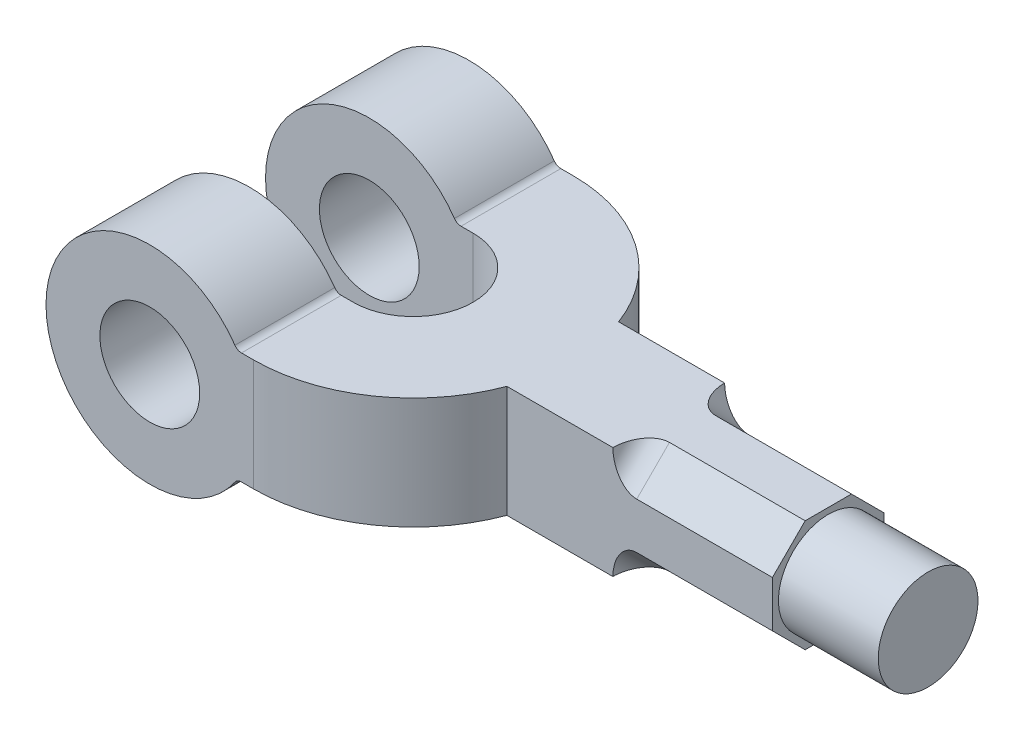
ISO-10303-21;
HEADER;
FILE_DESCRIPTION(('STEP AP214'),'2;1');
FILE_NAME('part.step','',(''),(''),'','','');
FILE_SCHEMA(('AUTOMOTIVE_DESIGN { 1 0 10303 214 1 1 1 1 }'));
ENDSEC;
DATA;
#1=APPLICATION_CONTEXT('core data for automotive mechanical design processes');
#2=APPLICATION_PROTOCOL_DEFINITION('international standard','automotive_design',2000,#1);
#3=PRODUCT_CONTEXT('',#1,'mechanical');
#4=PRODUCT('Part','Part','',(#3));
#5=PRODUCT_RELATED_PRODUCT_CATEGORY('part','',(#4));
#6=PRODUCT_DEFINITION_FORMATION('','',#4);
#7=PRODUCT_DEFINITION_CONTEXT('part definition',#1,'design');
#8=PRODUCT_DEFINITION('design','',#6,#7);
#9=PRODUCT_DEFINITION_SHAPE('','',#8);
#10=(LENGTH_UNIT() NAMED_UNIT(*) SI_UNIT(.MILLI.,.METRE.));
#11=(NAMED_UNIT(*) PLANE_ANGLE_UNIT() SI_UNIT($,.RADIAN.));
#12=(NAMED_UNIT(*) SI_UNIT($,.STERADIAN.) SOLID_ANGLE_UNIT());
#13=UNCERTAINTY_MEASURE_WITH_UNIT(LENGTH_MEASURE(1.E-05),#10,'distance_accuracy_value','');
#14=(GEOMETRIC_REPRESENTATION_CONTEXT(3) GLOBAL_UNCERTAINTY_ASSIGNED_CONTEXT((#13)) GLOBAL_UNIT_ASSIGNED_CONTEXT((#10,
#11,#12)) REPRESENTATION_CONTEXT('',''));
#15=CARTESIAN_POINT('',(0.,0.,0.));
#16=DIRECTION('',(0.,0.,1.));
#17=DIRECTION('',(1.,0.,0.));
#18=AXIS2_PLACEMENT_3D('',#15,#16,#17);
#19=CARTESIAN_POINT('',(-26.001,14.,-15.));
#20=DIRECTION('',(0.,-1.,0.));
#21=DIRECTION('',(0.,0.,-1.));
#22=AXIS2_PLACEMENT_3D('',#19,#20,#21);
#23=PLANE('',#22);
#24=DIRECTION('',(1.,0.,0.));
#25=VECTOR('',#24,1.);
#26=CARTESIAN_POINT('',(-26.001,14.,-40.));
#27=LINE('',#26,#25);
#28=CARTESIAN_POINT('',(22.9782505861521,14.,-40.));
#29=VERTEX_POINT('',#28);
#30=CARTESIAN_POINT('',(26.,14.,-40.));
#31=VERTEX_POINT('',#30);
#32=EDGE_CURVE('E276',#29,#31,#27,.T.);
#33=ORIENTED_EDGE('',*,*,#32,.F.);
#34=DIRECTION('',(0.,0.,1.));
#35=VECTOR('',#34,1.);
#36=CARTESIAN_POINT('',(22.9782505861521,14.,-15.));
#37=LINE('',#36,#35);
#38=CARTESIAN_POINT('',(22.9782505861521,14.,-15.));
#39=VERTEX_POINT('',#38);
#40=EDGE_CURVE('E344',#29,#39,#37,.T.);
#41=ORIENTED_EDGE('',*,*,#40,.T.);
#42=DIRECTION('',(1.,0.,0.));
#43=VECTOR('',#42,1.);
#44=CARTESIAN_POINT('',(-26.001,14.,-15.));
#45=LINE('',#44,#43);
#46=CARTESIAN_POINT('',(26.,14.,-15.));
#47=VERTEX_POINT('',#46);
#48=EDGE_CURVE('E274',#39,#47,#45,.T.);
#49=ORIENTED_EDGE('',*,*,#48,.T.);
#50=CARTESIAN_POINT('',(26.,14.,0.));
#51=DIRECTION('',(0.,-1.,0.));
#52=DIRECTION('',(0.,0.,1.));
#53=AXIS2_PLACEMENT_3D('',#50,#51,#52);
#54=CIRCLE('',#53,15.);
#55=CARTESIAN_POINT('',(26.,14.,15.));
#56=VERTEX_POINT('',#55);
#57=EDGE_CURVE('E238',#47,#56,#54,.T.);
#58=ORIENTED_EDGE('',*,*,#57,.T.);
#59=DIRECTION('',(1.,0.,0.));
#60=VECTOR('',#59,1.);
#61=CARTESIAN_POINT('',(-26.001,14.,15.));
#62=LINE('',#61,#60);
#63=CARTESIAN_POINT('',(22.9782505861521,14.,15.));
#64=VERTEX_POINT('',#63);
#65=EDGE_CURVE('E414',#64,#56,#62,.T.);
#66=ORIENTED_EDGE('',*,*,#65,.F.);
#67=DIRECTION('',(0.,0.,1.));
#68=VECTOR('',#67,1.);
#69=CARTESIAN_POINT('',(22.9782505861521,14.,40.));
#70=LINE('',#69,#68);
#71=CARTESIAN_POINT('',(22.9782505861521,14.,40.));
#72=VERTEX_POINT('',#71);
#73=EDGE_CURVE('E54',#64,#72,#70,.T.);
#74=ORIENTED_EDGE('',*,*,#73,.T.);
#75=DIRECTION('',(1.,0.,0.));
#76=VECTOR('',#75,1.);
#77=CARTESIAN_POINT('',(-26.001,14.,40.));
#78=LINE('',#77,#76);
#79=CARTESIAN_POINT('',(26.,14.,40.));
#80=VERTEX_POINT('',#79);
#81=EDGE_CURVE('E246',#72,#80,#78,.T.);
#82=ORIENTED_EDGE('',*,*,#81,.T.);
#83=CARTESIAN_POINT('',(26.,14.,0.));
#84=DIRECTION('',(0.,1.,0.));
#85=DIRECTION('',(0.,0.,1.));
#86=AXIS2_PLACEMENT_3D('',#83,#84,#85);
#87=CIRCLE('',#86,40.);
#88=CARTESIAN_POINT('',(63.4699879903904,14.,14.));
#89=VERTEX_POINT('',#88);
#90=EDGE_CURVE('E235',#80,#89,#87,.T.);
#91=ORIENTED_EDGE('',*,*,#90,.T.);
#92=DIRECTION('',(1.,0.,0.));
#93=VECTOR('',#92,1.);
#94=CARTESIAN_POINT('',(130.,14.,14.));
#95=LINE('',#94,#93);
#96=CARTESIAN_POINT('',(90.0033680345603,14.,14.));
#97=VERTEX_POINT('',#96);
#98=EDGE_CURVE('E226',#89,#97,#95,.T.);
#99=ORIENTED_EDGE('',*,*,#98,.T.);
#100=CARTESIAN_POINT('',(96.,14.,14.2842712474619));
#101=DIRECTION('',(0.,-1.,0.));
#102=DIRECTION('',(0.,0.,-1.));
#103=AXIS2_PLACEMENT_3D('',#100,#101,#102);
#104=ELLIPSE('',#103,8.48528137423856,6.);
#105=CARTESIAN_POINT('',(96.,14.,5.79898987322334));
#106=VERTEX_POINT('',#105);
#107=EDGE_CURVE('E319',#97,#106,#104,.T.);
#108=ORIENTED_EDGE('',*,*,#107,.T.);
#109=DIRECTION('',(1.,0.,0.));
#110=VECTOR('',#109,1.);
#111=CARTESIAN_POINT('',(90.,14.,5.79898987322334));
#112=LINE('',#111,#110);
#113=CARTESIAN_POINT('',(130.,14.,5.79898987322334));
#114=VERTEX_POINT('',#113);
#115=EDGE_CURVE('E208',#106,#114,#112,.T.);
#116=ORIENTED_EDGE('',*,*,#115,.T.);
#117=DIRECTION('',(0.,0.,-1.));
#118=VECTOR('',#117,1.);
#119=CARTESIAN_POINT('',(130.,14.,-14.));
#120=LINE('',#119,#118);
#121=CARTESIAN_POINT('',(130.,14.,-5.79898987322332));
#122=VERTEX_POINT('',#121);
#123=EDGE_CURVE('E219',#114,#122,#120,.T.);
#124=ORIENTED_EDGE('',*,*,#123,.T.);
#125=DIRECTION('',(1.,0.,0.));
#126=VECTOR('',#125,1.);
#127=CARTESIAN_POINT('',(90.,14.,-5.79898987322332));
#128=LINE('',#127,#126);
#129=CARTESIAN_POINT('',(96.,14.,-5.79898987322332));
#130=VERTEX_POINT('',#129);
#131=EDGE_CURVE('E200',#130,#122,#128,.T.);
#132=ORIENTED_EDGE('',*,*,#131,.F.);
#133=CARTESIAN_POINT('',(96.,14.,-14.2842712474619));
#134=DIRECTION('',(0.,-1.,0.));
#135=DIRECTION('',(0.,0.,-1.));
#136=AXIS2_PLACEMENT_3D('',#133,#134,#135);
#137=ELLIPSE('',#136,8.48528137423857,6.);
#138=CARTESIAN_POINT('',(90.0033680345603,14.,-14.));
#139=VERTEX_POINT('',#138);
#140=EDGE_CURVE('E311',#130,#139,#137,.T.);
#141=ORIENTED_EDGE('',*,*,#140,.T.);
#142=DIRECTION('',(-1.,0.,0.));
#143=VECTOR('',#142,1.);
#144=CARTESIAN_POINT('',(130.,14.,-14.));
#145=LINE('',#144,#143);
#146=CARTESIAN_POINT('',(63.4699879903904,14.,-14.));
#147=VERTEX_POINT('',#146);
#148=EDGE_CURVE('E227',#139,#147,#145,.T.);
#149=ORIENTED_EDGE('',*,*,#148,.T.);
#150=CARTESIAN_POINT('',(26.,14.,0.));
#151=DIRECTION('',(0.,1.,0.));
#152=DIRECTION('',(0.,0.,1.));
#153=AXIS2_PLACEMENT_3D('',#150,#151,#152);
#154=CIRCLE('',#153,40.);
#155=EDGE_CURVE('E229',#147,#31,#154,.T.);
#156=ORIENTED_EDGE('',*,*,#155,.T.);
#157=EDGE_LOOP('',(#33,#41,#49,#58,#66,#74,#82,#91,#99,#108,#116,#124,#132,#141,#149,#156));
#158=FACE_BOUND('',#157,.T.);
#159=ADVANCED_FACE('F37',(#158),#23,.F.);
#160=CARTESIAN_POINT('',(130.,14.,14.));
#161=DIRECTION('',(0.,0.,-1.));
#162=DIRECTION('',(-1.,0.,0.));
#163=AXIS2_PLACEMENT_3D('',#160,#161,#162);
#164=PLANE('',#163);
#165=DIRECTION('',(1.,0.,0.));
#166=VECTOR('',#165,1.);
#167=CARTESIAN_POINT('',(130.,-14.,14.));
#168=LINE('',#167,#166);
#169=CARTESIAN_POINT('',(63.4699879903904,-14.,14.));
#170=VERTEX_POINT('',#169);
#171=CARTESIAN_POINT('',(90.0033680345603,-14.,14.));
#172=VERTEX_POINT('',#171);
#173=EDGE_CURVE('E244',#170,#172,#168,.T.);
#174=ORIENTED_EDGE('',*,*,#173,.T.);
#175=CARTESIAN_POINT('',(96.,-14.2842712474619,14.));
#176=DIRECTION('',(0.,0.,-1.));
#177=DIRECTION('',(0.,1.,0.));
#178=AXIS2_PLACEMENT_3D('',#175,#176,#177);
#179=ELLIPSE('',#178,8.48528137423857,6.);
#180=CARTESIAN_POINT('',(96.,-5.79898987322333,14.));
#181=VERTEX_POINT('',#180);
#182=EDGE_CURVE('E324',#172,#181,#179,.T.);
#183=ORIENTED_EDGE('',*,*,#182,.T.);
#184=DIRECTION('',(1.,0.,0.));
#185=VECTOR('',#184,1.);
#186=CARTESIAN_POINT('',(90.,-5.79898987322333,14.));
#187=LINE('',#186,#185);
#188=CARTESIAN_POINT('',(130.,-5.79898987322333,14.));
#189=VERTEX_POINT('',#188);
#190=EDGE_CURVE('E432',#181,#189,#187,.T.);
#191=ORIENTED_EDGE('',*,*,#190,.T.);
#192=DIRECTION('',(0.,-1.,0.));
#193=VECTOR('',#192,1.);
#194=CARTESIAN_POINT('',(130.,14.,14.));
#195=LINE('',#194,#193);
#196=CARTESIAN_POINT('',(130.,5.79898987322333,14.));
#197=VERTEX_POINT('',#196);
#198=EDGE_CURVE('E269',#197,#189,#195,.T.);
#199=ORIENTED_EDGE('',*,*,#198,.F.);
#200=DIRECTION('',(1.,0.,0.));
#201=VECTOR('',#200,1.);
#202=CARTESIAN_POINT('',(90.,5.79898987322332,14.));
#203=LINE('',#202,#201);
#204=CARTESIAN_POINT('',(96.,5.79898987322332,14.));
#205=VERTEX_POINT('',#204);
#206=EDGE_CURVE('E430',#205,#197,#203,.T.);
#207=ORIENTED_EDGE('',*,*,#206,.F.);
#208=CARTESIAN_POINT('',(96.,14.2842712474619,14.));
#209=DIRECTION('',(0.,0.,-1.));
#210=DIRECTION('',(0.,1.,0.));
#211=AXIS2_PLACEMENT_3D('',#208,#209,#210);
#212=ELLIPSE('',#211,8.48528137423857,6.);
#213=EDGE_CURVE('E314',#205,#97,#212,.T.);
#214=ORIENTED_EDGE('',*,*,#213,.T.);
#215=ORIENTED_EDGE('',*,*,#98,.F.);
#216=DIRECTION('',(0.,-1.,0.));
#217=VECTOR('',#216,1.);
#218=CARTESIAN_POINT('',(63.4699879903904,14.,14.));
#219=LINE('',#218,#217);
#220=EDGE_CURVE('E272',#89,#170,#219,.T.);
#221=ORIENTED_EDGE('',*,*,#220,.T.);
#222=EDGE_LOOP('',(#174,#183,#191,#199,#207,#214,#215,#221));
#223=FACE_BOUND('',#222,.T.);
#224=ADVANCED_FACE('F421',(#223),#164,.F.);
#225=CARTESIAN_POINT('',(130.,14.,-14.));
#226=DIRECTION('',(-1.,0.,0.));
#227=DIRECTION('',(0.,0.,1.));
#228=AXIS2_PLACEMENT_3D('',#225,#226,#227);
#229=PLANE('',#228);
#230=CARTESIAN_POINT('',(130.,0.,0.));
#231=DIRECTION('',(1.,0.,0.));
#232=DIRECTION('',(0.,0.,-1.));
#233=AXIS2_PLACEMENT_3D('',#230,#231,#232);
#234=CIRCLE('',#233,12.5);
#235=CARTESIAN_POINT('',(130.,0.,-12.5));
#236=VERTEX_POINT('',#235);
#237=EDGE_CURVE('E323',#236,#236,#234,.T.);
#238=ORIENTED_EDGE('',*,*,#237,.F.);
#239=EDGE_LOOP('',(#238));
#240=FACE_BOUND('',#239,.T.);
#241=DIRECTION('',(0.,0.707106781186548,-0.707106781186547));
#242=VECTOR('',#241,1.);
#243=CARTESIAN_POINT('',(130.,-14.,-5.79898987322333));
#244=LINE('',#243,#242);
#245=CARTESIAN_POINT('',(130.,-14.,-5.79898987322333));
#246=VERTEX_POINT('',#245);
#247=CARTESIAN_POINT('',(130.,-5.79898987322332,-14.));
#248=VERTEX_POINT('',#247);
#249=EDGE_CURVE('E225',#246,#248,#244,.T.);
#250=ORIENTED_EDGE('',*,*,#249,.T.);
#251=DIRECTION('',(0.,-1.,0.));
#252=VECTOR('',#251,1.);
#253=CARTESIAN_POINT('',(130.,14.,-14.));
#254=LINE('',#253,#252);
#255=CARTESIAN_POINT('',(130.,5.79898987322333,-14.));
#256=VERTEX_POINT('',#255);
#257=EDGE_CURVE('E220',#256,#248,#254,.T.);
#258=ORIENTED_EDGE('',*,*,#257,.F.);
#259=DIRECTION('',(0.,0.707106781186547,0.707106781186548));
#260=VECTOR('',#259,1.);
#261=CARTESIAN_POINT('',(130.,5.79898987322333,-14.));
#262=LINE('',#261,#260);
#263=EDGE_CURVE('E201',#256,#122,#262,.T.);
#264=ORIENTED_EDGE('',*,*,#263,.T.);
#265=ORIENTED_EDGE('',*,*,#123,.F.);
#266=DIRECTION('',(0.,-0.707106781186548,0.707106781186547));
#267=VECTOR('',#266,1.);
#268=CARTESIAN_POINT('',(130.,14.,5.79898987322334));
#269=LINE('',#268,#267);
#270=EDGE_CURVE('E222',#114,#197,#269,.T.);
#271=ORIENTED_EDGE('',*,*,#270,.T.);
#272=ORIENTED_EDGE('',*,*,#198,.T.);
#273=DIRECTION('',(0.,-0.707106781186547,-0.707106781186548));
#274=VECTOR('',#273,1.);
#275=CARTESIAN_POINT('',(130.,-5.79898987322333,14.));
#276=LINE('',#275,#274);
#277=CARTESIAN_POINT('',(130.,-14.,5.79898987322333));
#278=VERTEX_POINT('',#277);
#279=EDGE_CURVE('E437',#189,#278,#276,.T.);
#280=ORIENTED_EDGE('',*,*,#279,.T.);
#281=DIRECTION('',(0.,0.,-1.));
#282=VECTOR('',#281,1.);
#283=CARTESIAN_POINT('',(130.,-14.,-14.));
#284=LINE('',#283,#282);
#285=EDGE_CURVE('E247',#278,#246,#284,.T.);
#286=ORIENTED_EDGE('',*,*,#285,.T.);
#287=EDGE_LOOP('',(#250,#258,#264,#265,#271,#272,#280,#286));
#288=FACE_BOUND('',#287,.T.);
#289=ADVANCED_FACE('F216',(#240,#288),#229,.F.);
#290=CARTESIAN_POINT('',(130.,14.,-14.));
#291=DIRECTION('',(0.,0.,1.));
#292=DIRECTION('',(1.,0.,0.));
#293=AXIS2_PLACEMENT_3D('',#290,#291,#292);
#294=PLANE('',#293);
#295=DIRECTION('',(1.,0.,0.));
#296=VECTOR('',#295,1.);
#297=CARTESIAN_POINT('',(90.,-5.79898987322332,-14.));
#298=LINE('',#297,#296);
#299=CARTESIAN_POINT('',(96.,-5.79898987322332,-14.));
#300=VERTEX_POINT('',#299);
#301=EDGE_CURVE('E438',#300,#248,#298,.T.);
#302=ORIENTED_EDGE('',*,*,#301,.F.);
#303=CARTESIAN_POINT('',(96.,-14.2842712474619,-14.));
#304=DIRECTION('',(0.,0.,1.));
#305=DIRECTION('',(0.,-1.,0.));
#306=AXIS2_PLACEMENT_3D('',#303,#304,#305);
#307=ELLIPSE('',#306,8.48528137423857,6.);
#308=CARTESIAN_POINT('',(90.0033680345603,-14.,-14.));
#309=VERTEX_POINT('',#308);
#310=EDGE_CURVE('E306',#300,#309,#307,.T.);
#311=ORIENTED_EDGE('',*,*,#310,.T.);
#312=DIRECTION('',(-1.,0.,0.));
#313=VECTOR('',#312,1.);
#314=CARTESIAN_POINT('',(130.,-14.,-14.));
#315=LINE('',#314,#313);
#316=CARTESIAN_POINT('',(63.4699879903904,-14.,-14.));
#317=VERTEX_POINT('',#316);
#318=EDGE_CURVE('E252',#309,#317,#315,.T.);
#319=ORIENTED_EDGE('',*,*,#318,.T.);
#320=DIRECTION('',(0.,-1.,0.));
#321=VECTOR('',#320,1.);
#322=CARTESIAN_POINT('',(63.4699879903904,14.,-14.));
#323=LINE('',#322,#321);
#324=EDGE_CURVE('E263',#147,#317,#323,.T.);
#325=ORIENTED_EDGE('',*,*,#324,.F.);
#326=ORIENTED_EDGE('',*,*,#148,.F.);
#327=CARTESIAN_POINT('',(96.,14.2842712474619,-14.));
#328=DIRECTION('',(0.,0.,1.));
#329=DIRECTION('',(0.,-1.,0.));
#330=AXIS2_PLACEMENT_3D('',#327,#328,#329);
#331=ELLIPSE('',#330,8.48528137423857,6.);
#332=CARTESIAN_POINT('',(96.,5.79898987322333,-14.));
#333=VERTEX_POINT('',#332);
#334=EDGE_CURVE('E312',#139,#333,#331,.T.);
#335=ORIENTED_EDGE('',*,*,#334,.T.);
#336=DIRECTION('',(1.,0.,0.));
#337=VECTOR('',#336,1.);
#338=CARTESIAN_POINT('',(90.,5.79898987322333,-14.));
#339=LINE('',#338,#337);
#340=EDGE_CURVE('E212',#333,#256,#339,.T.);
#341=ORIENTED_EDGE('',*,*,#340,.T.);
#342=ORIENTED_EDGE('',*,*,#257,.T.);
#343=EDGE_LOOP('',(#302,#311,#319,#325,#326,#335,#341,#342));
#344=FACE_BOUND('',#343,.T.);
#345=ADVANCED_FACE('F458',(#344),#294,.F.);
#346=CARTESIAN_POINT('',(26.,-14.,0.));
#347=DIRECTION('',(0.,1.,0.));
#348=DIRECTION('',(0.,0.,1.));
#349=AXIS2_PLACEMENT_3D('',#346,#347,#348);
#350=PLANE('',#349);
#351=DIRECTION('',(1.,0.,0.));
#352=VECTOR('',#351,1.);
#353=CARTESIAN_POINT('',(-26.001,-14.,-15.));
#354=LINE('',#353,#352);
#355=CARTESIAN_POINT('',(22.9782505861521,-14.,-15.));
#356=VERTEX_POINT('',#355);
#357=CARTESIAN_POINT('',(26.,-14.,-15.));
#358=VERTEX_POINT('',#357);
#359=EDGE_CURVE('E384',#356,#358,#354,.T.);
#360=ORIENTED_EDGE('',*,*,#359,.F.);
#361=DIRECTION('',(0.,0.,1.));
#362=VECTOR('',#361,1.);
#363=CARTESIAN_POINT('',(22.9782505861521,-14.,-40.));
#364=LINE('',#363,#362);
#365=CARTESIAN_POINT('',(22.9782505861521,-14.,-40.));
#366=VERTEX_POINT('',#365);
#367=EDGE_CURVE('E331',#356,#366,#364,.F.);
#368=ORIENTED_EDGE('',*,*,#367,.T.);
#369=DIRECTION('',(1.,0.,0.));
#370=VECTOR('',#369,1.);
#371=CARTESIAN_POINT('',(-26.001,-14.,-40.));
#372=LINE('',#371,#370);
#373=CARTESIAN_POINT('',(26.,-14.,-40.));
#374=VERTEX_POINT('',#373);
#375=EDGE_CURVE('E378',#366,#374,#372,.T.);
#376=ORIENTED_EDGE('',*,*,#375,.T.);
#377=CARTESIAN_POINT('',(26.,-14.,0.));
#378=DIRECTION('',(0.,1.,0.));
#379=DIRECTION('',(0.,0.,1.));
#380=AXIS2_PLACEMENT_3D('',#377,#378,#379);
#381=CIRCLE('',#380,40.);
#382=EDGE_CURVE('E254',#317,#374,#381,.T.);
#383=ORIENTED_EDGE('',*,*,#382,.F.);
#384=ORIENTED_EDGE('',*,*,#318,.F.);
#385=CARTESIAN_POINT('',(96.,-14.,-14.2842712474619));
#386=DIRECTION('',(0.,1.,0.));
#387=DIRECTION('',(0.,0.,1.));
#388=AXIS2_PLACEMENT_3D('',#385,#386,#387);
#389=ELLIPSE('',#388,8.48528137423857,6.);
#390=CARTESIAN_POINT('',(96.,-14.,-5.79898987322333));
#391=VERTEX_POINT('',#390);
#392=EDGE_CURVE('E307',#309,#391,#389,.T.);
#393=ORIENTED_EDGE('',*,*,#392,.T.);
#394=DIRECTION('',(1.,0.,0.));
#395=VECTOR('',#394,1.);
#396=CARTESIAN_POINT('',(90.,-14.,-5.79898987322333));
#397=LINE('',#396,#395);
#398=EDGE_CURVE('E392',#391,#246,#397,.T.);
#399=ORIENTED_EDGE('',*,*,#398,.T.);
#400=ORIENTED_EDGE('',*,*,#285,.F.);
#401=DIRECTION('',(1.,0.,0.));
#402=VECTOR('',#401,1.);
#403=CARTESIAN_POINT('',(90.,-14.,5.79898987322333));
#404=LINE('',#403,#402);
#405=CARTESIAN_POINT('',(96.,-14.,5.79898987322333));
#406=VERTEX_POINT('',#405);
#407=EDGE_CURVE('E393',#406,#278,#404,.T.);
#408=ORIENTED_EDGE('',*,*,#407,.F.);
#409=CARTESIAN_POINT('',(96.,-14.,14.2842712474619));
#410=DIRECTION('',(0.,1.,0.));
#411=DIRECTION('',(0.,0.,1.));
#412=AXIS2_PLACEMENT_3D('',#409,#410,#411);
#413=ELLIPSE('',#412,8.48528137423857,6.);
#414=EDGE_CURVE('E318',#406,#172,#413,.T.);
#415=ORIENTED_EDGE('',*,*,#414,.T.);
#416=ORIENTED_EDGE('',*,*,#173,.F.);
#417=CARTESIAN_POINT('',(26.,-14.,0.));
#418=DIRECTION('',(0.,1.,0.));
#419=DIRECTION('',(0.,0.,1.));
#420=AXIS2_PLACEMENT_3D('',#417,#418,#419);
#421=CIRCLE('',#420,40.);
#422=CARTESIAN_POINT('',(26.,-14.,40.));
#423=VERTEX_POINT('',#422);
#424=EDGE_CURVE('E245',#423,#170,#421,.T.);
#425=ORIENTED_EDGE('',*,*,#424,.F.);
#426=DIRECTION('',(1.,0.,0.));
#427=VECTOR('',#426,1.);
#428=CARTESIAN_POINT('',(-26.001,-14.,40.));
#429=LINE('',#428,#427);
#430=CARTESIAN_POINT('',(22.9782505861521,-14.,40.));
#431=VERTEX_POINT('',#430);
#432=EDGE_CURVE('E385',#431,#423,#429,.T.);
#433=ORIENTED_EDGE('',*,*,#432,.F.);
#434=DIRECTION('',(0.,0.,1.));
#435=VECTOR('',#434,1.);
#436=CARTESIAN_POINT('',(22.9782505861521,-14.,15.));
#437=LINE('',#436,#435);
#438=CARTESIAN_POINT('',(22.9782505861521,-14.,15.));
#439=VERTEX_POINT('',#438);
#440=EDGE_CURVE('E335',#431,#439,#437,.F.);
#441=ORIENTED_EDGE('',*,*,#440,.T.);
#442=DIRECTION('',(1.,0.,0.));
#443=VECTOR('',#442,1.);
#444=CARTESIAN_POINT('',(-26.001,-14.,15.));
#445=LINE('',#444,#443);
#446=CARTESIAN_POINT('',(26.,-14.,15.));
#447=VERTEX_POINT('',#446);
#448=EDGE_CURVE('E399',#439,#447,#445,.T.);
#449=ORIENTED_EDGE('',*,*,#448,.T.);
#450=CARTESIAN_POINT('',(26.,-14.,0.));
#451=DIRECTION('',(0.,-1.,0.));
#452=DIRECTION('',(0.,0.,1.));
#453=AXIS2_PLACEMENT_3D('',#450,#451,#452);
#454=CIRCLE('',#453,15.);
#455=EDGE_CURVE('E257',#358,#447,#454,.T.);
#456=ORIENTED_EDGE('',*,*,#455,.F.);
#457=EDGE_LOOP('',(#360,#368,#376,#383,#384,#393,#399,#400,#408,#415,#416,#425,#433,#441,#449,#456));
#458=FACE_BOUND('',#457,.T.);
#459=ADVANCED_FACE('F391',(#458),#350,.F.);
#460=CARTESIAN_POINT('',(0.,0.,40.));
#461=DIRECTION('',(0.,0.,-1.));
#462=DIRECTION('',(-1.,0.,0.));
#463=AXIS2_PLACEMENT_3D('',#460,#461,#462);
#464=CYLINDRICAL_SURFACE('',#463,26.);
#465=CARTESIAN_POINT('',(0.,0.,-40.));
#466=DIRECTION('',(0.,0.,1.));
#467=DIRECTION('',(1.,0.,0.));
#468=AXIS2_PLACEMENT_3D('',#465,#466,#467);
#469=CIRCLE('',#468,26.);
#470=CARTESIAN_POINT('',(21.3369469728555,14.8571428571429,-40.));
#471=VERTEX_POINT('',#470);
#472=CARTESIAN_POINT('',(21.3369469728555,-14.8571428571429,-40.));
#473=VERTEX_POINT('',#472);
#474=EDGE_CURVE('E279',#471,#473,#469,.T.);
#475=ORIENTED_EDGE('',*,*,#474,.T.);
#476=DIRECTION('',(0.,0.,-1.));
#477=VECTOR('',#476,1.);
#478=CARTESIAN_POINT('',(21.3369469728555,-14.8571428571429,40.));
#479=LINE('',#478,#477);
#480=CARTESIAN_POINT('',(21.3369469728555,-14.8571428571429,-15.));
#481=VERTEX_POINT('',#480);
#482=EDGE_CURVE('E328',#473,#481,#479,.F.);
#483=ORIENTED_EDGE('',*,*,#482,.T.);
#484=CARTESIAN_POINT('',(0.,0.,-15.));
#485=DIRECTION('',(0.,0.,1.));
#486=DIRECTION('',(1.,0.,0.));
#487=AXIS2_PLACEMENT_3D('',#484,#485,#486);
#488=CIRCLE('',#487,26.);
#489=CARTESIAN_POINT('',(21.3369469728555,14.8571428571429,-15.));
#490=VERTEX_POINT('',#489);
#491=EDGE_CURVE('E293',#490,#481,#488,.T.);
#492=ORIENTED_EDGE('',*,*,#491,.F.);
#493=DIRECTION('',(0.,0.,-1.));
#494=VECTOR('',#493,1.);
#495=CARTESIAN_POINT('',(21.3369469728555,14.8571428571429,40.));
#496=LINE('',#495,#494);
#497=EDGE_CURVE('E326',#490,#471,#496,.T.);
#498=ORIENTED_EDGE('',*,*,#497,.T.);
#499=EDGE_LOOP('',(#475,#483,#492,#498));
#500=FACE_BOUND('',#499,.T.);
#501=ADVANCED_FACE('F362',(#500),#464,.T.);
#502=CARTESIAN_POINT('',(0.,0.,40.));
#503=DIRECTION('',(0.,0.,-1.));
#504=DIRECTION('',(-1.,0.,0.));
#505=AXIS2_PLACEMENT_3D('',#502,#503,#504);
#506=CYLINDRICAL_SURFACE('',#505,26.);
#507=CARTESIAN_POINT('',(0.,0.,15.));
#508=DIRECTION('',(0.,0.,1.));
#509=DIRECTION('',(1.,0.,0.));
#510=AXIS2_PLACEMENT_3D('',#507,#508,#509);
#511=CIRCLE('',#510,26.);
#512=CARTESIAN_POINT('',(21.3369469728555,14.8571428571429,15.));
#513=VERTEX_POINT('',#512);
#514=CARTESIAN_POINT('',(21.3369469728555,-14.8571428571429,15.));
#515=VERTEX_POINT('',#514);
#516=EDGE_CURVE('E404',#513,#515,#511,.T.);
#517=ORIENTED_EDGE('',*,*,#516,.T.);
#518=DIRECTION('',(0.,0.,-1.));
#519=VECTOR('',#518,1.);
#520=CARTESIAN_POINT('',(21.3369469728555,-14.8571428571429,40.));
#521=LINE('',#520,#519);
#522=CARTESIAN_POINT('',(21.3369469728555,-14.8571428571429,40.));
#523=VERTEX_POINT('',#522);
#524=EDGE_CURVE('E339',#515,#523,#521,.F.);
#525=ORIENTED_EDGE('',*,*,#524,.T.);
#526=CARTESIAN_POINT('',(0.,0.,40.));
#527=DIRECTION('',(0.,0.,1.));
#528=DIRECTION('',(1.,0.,0.));
#529=AXIS2_PLACEMENT_3D('',#526,#527,#528);
#530=CIRCLE('',#529,26.);
#531=CARTESIAN_POINT('',(21.3369469728555,14.8571428571429,40.));
#532=VERTEX_POINT('',#531);
#533=EDGE_CURVE('E408',#532,#523,#530,.T.);
#534=ORIENTED_EDGE('',*,*,#533,.F.);
#535=DIRECTION('',(0.,0.,-1.));
#536=VECTOR('',#535,1.);
#537=CARTESIAN_POINT('',(21.3369469728555,14.8571428571429,40.));
#538=LINE('',#537,#536);
#539=EDGE_CURVE('E337',#532,#513,#538,.T.);
#540=ORIENTED_EDGE('',*,*,#539,.T.);
#541=EDGE_LOOP('',(#517,#525,#534,#540));
#542=FACE_BOUND('',#541,.T.);
#543=ADVANCED_FACE('F495',(#542),#506,.T.);
#544=CARTESIAN_POINT('',(0.,0.,40.));
#545=DIRECTION('',(0.,0.,-1.));
#546=DIRECTION('',(-1.,0.,0.));
#547=AXIS2_PLACEMENT_3D('',#544,#545,#546);
#548=CYLINDRICAL_SURFACE('',#547,12.5);
#549=CARTESIAN_POINT('',(0.,0.,-40.));
#550=DIRECTION('',(0.,0.,1.));
#551=DIRECTION('',(1.,0.,0.));
#552=AXIS2_PLACEMENT_3D('',#549,#550,#551);
#553=CIRCLE('',#552,12.5);
#554=CARTESIAN_POINT('',(12.5,0.,-40.));
#555=VERTEX_POINT('',#554);
#556=EDGE_CURVE('E289',#555,#555,#553,.T.);
#557=ORIENTED_EDGE('',*,*,#556,.F.);
#558=EDGE_LOOP('',(#557));
#559=FACE_BOUND('',#558,.T.);
#560=CARTESIAN_POINT('',(0.,0.,-15.));
#561=DIRECTION('',(0.,0.,1.));
#562=DIRECTION('',(1.,0.,0.));
#563=AXIS2_PLACEMENT_3D('',#560,#561,#562);
#564=CIRCLE('',#563,12.5);
#565=CARTESIAN_POINT('',(12.5,0.,-15.));
#566=VERTEX_POINT('',#565);
#567=EDGE_CURVE('E290',#566,#566,#564,.T.);
#568=ORIENTED_EDGE('',*,*,#567,.T.);
#569=EDGE_LOOP('',(#568));
#570=FACE_BOUND('',#569,.T.);
#571=ADVANCED_FACE('F488',(#559,#570),#548,.F.);
#572=CARTESIAN_POINT('',(0.,0.,-40.));
#573=DIRECTION('',(0.,0.,1.));
#574=DIRECTION('',(1.,0.,0.));
#575=AXIS2_PLACEMENT_3D('',#572,#573,#574);
#576=PLANE('',#575);
#577=ORIENTED_EDGE('',*,*,#474,.F.);
#578=CARTESIAN_POINT('',(22.9782505861521,16.,-40.));
#579=DIRECTION('',(0.,0.,1.));
#580=DIRECTION('',(1.,0.,0.));
#581=AXIS2_PLACEMENT_3D('',#578,#579,#580);
#582=CIRCLE('',#581,2.);
#583=EDGE_CURVE('E354',#471,#29,#582,.T.);
#584=ORIENTED_EDGE('',*,*,#583,.T.);
#585=ORIENTED_EDGE('',*,*,#32,.T.);
#586=DIRECTION('',(0.,-1.,0.));
#587=VECTOR('',#586,1.);
#588=CARTESIAN_POINT('',(26.,14.,-40.));
#589=LINE('',#588,#587);
#590=EDGE_CURVE('E273',#31,#374,#589,.T.);
#591=ORIENTED_EDGE('',*,*,#590,.T.);
#592=ORIENTED_EDGE('',*,*,#375,.F.);
#593=CARTESIAN_POINT('',(22.9782505861521,-16.,-40.));
#594=DIRECTION('',(0.,0.,1.));
#595=DIRECTION('',(1.,0.,0.));
#596=AXIS2_PLACEMENT_3D('',#593,#594,#595);
#597=CIRCLE('',#596,2.);
#598=EDGE_CURVE('E347',#366,#473,#597,.T.);
#599=ORIENTED_EDGE('',*,*,#598,.T.);
#600=EDGE_LOOP('',(#577,#584,#585,#591,#592,#599));
#601=FACE_BOUND('',#600,.T.);
#602=ORIENTED_EDGE('',*,*,#556,.T.);
#603=EDGE_LOOP('',(#602));
#604=FACE_BOUND('',#603,.T.);
#605=ADVANCED_FACE('F369',(#601,#604),#576,.F.);
#606=CARTESIAN_POINT('',(0.,0.,-15.));
#607=DIRECTION('',(0.,0.,1.));
#608=DIRECTION('',(1.,0.,0.));
#609=AXIS2_PLACEMENT_3D('',#606,#607,#608);
#610=PLANE('',#609);
#611=ORIENTED_EDGE('',*,*,#567,.F.);
#612=EDGE_LOOP('',(#611));
#613=FACE_BOUND('',#612,.T.);
#614=ORIENTED_EDGE('',*,*,#48,.F.);
#615=CARTESIAN_POINT('',(22.9782505861521,16.,-15.));
#616=DIRECTION('',(0.,0.,1.));
#617=DIRECTION('',(1.,0.,0.));
#618=AXIS2_PLACEMENT_3D('',#615,#616,#617);
#619=CIRCLE('',#618,2.);
#620=EDGE_CURVE('E353',#39,#490,#619,.F.);
#621=ORIENTED_EDGE('',*,*,#620,.T.);
#622=ORIENTED_EDGE('',*,*,#491,.T.);
#623=CARTESIAN_POINT('',(22.9782505861521,-16.,-15.));
#624=DIRECTION('',(0.,0.,1.));
#625=DIRECTION('',(1.,0.,0.));
#626=AXIS2_PLACEMENT_3D('',#623,#624,#625);
#627=CIRCLE('',#626,2.);
#628=EDGE_CURVE('E343',#481,#356,#627,.F.);
#629=ORIENTED_EDGE('',*,*,#628,.T.);
#630=ORIENTED_EDGE('',*,*,#359,.T.);
#631=DIRECTION('',(0.,1.,0.));
#632=VECTOR('',#631,1.);
#633=CARTESIAN_POINT('',(26.,-14.,-15.));
#634=LINE('',#633,#632);
#635=EDGE_CURVE('E281',#358,#47,#634,.T.);
#636=ORIENTED_EDGE('',*,*,#635,.T.);
#637=EDGE_LOOP('',(#614,#621,#622,#629,#630,#636));
#638=FACE_BOUND('',#637,.T.);
#639=ADVANCED_FACE('F359',(#613,#638),#610,.T.);
#640=CARTESIAN_POINT('',(26.,14.,0.));
#641=DIRECTION('',(0.,-1.,0.));
#642=DIRECTION('',(0.,0.,-1.));
#643=AXIS2_PLACEMENT_3D('',#640,#641,#642);
#644=CYLINDRICAL_SURFACE('',#643,40.);
#645=ORIENTED_EDGE('',*,*,#424,.T.);
#646=ORIENTED_EDGE('',*,*,#220,.F.);
#647=ORIENTED_EDGE('',*,*,#90,.F.);
#648=DIRECTION('',(0.,-1.,0.));
#649=VECTOR('',#648,1.);
#650=CARTESIAN_POINT('',(26.,14.,40.));
#651=LINE('',#650,#649);
#652=EDGE_CURVE('E241',#80,#423,#651,.T.);
#653=ORIENTED_EDGE('',*,*,#652,.T.);
#654=EDGE_LOOP('',(#645,#646,#647,#653));
#655=FACE_BOUND('',#654,.T.);
#656=ADVANCED_FACE('F418',(#655),#644,.T.);
#657=CARTESIAN_POINT('',(26.,14.,0.));
#658=DIRECTION('',(0.,-1.,0.));
#659=DIRECTION('',(0.,0.,-1.));
#660=AXIS2_PLACEMENT_3D('',#657,#658,#659);
#661=CYLINDRICAL_SURFACE('',#660,40.);
#662=ORIENTED_EDGE('',*,*,#382,.T.);
#663=ORIENTED_EDGE('',*,*,#590,.F.);
#664=ORIENTED_EDGE('',*,*,#155,.F.);
#665=ORIENTED_EDGE('',*,*,#324,.T.);
#666=EDGE_LOOP('',(#662,#663,#664,#665));
#667=FACE_BOUND('',#666,.T.);
#668=ADVANCED_FACE('F376',(#667),#661,.T.);
#669=CARTESIAN_POINT('',(26.,14.,0.));
#670=DIRECTION('',(0.,-1.,0.));
#671=DIRECTION('',(0.,0.,-1.));
#672=AXIS2_PLACEMENT_3D('',#669,#670,#671);
#673=CYLINDRICAL_SURFACE('',#672,15.);
#674=ORIENTED_EDGE('',*,*,#455,.T.);
#675=DIRECTION('',(0.,-1.,0.));
#676=VECTOR('',#675,1.);
#677=CARTESIAN_POINT('',(26.,14.,15.));
#678=LINE('',#677,#676);
#679=EDGE_CURVE('E261',#56,#447,#678,.T.);
#680=ORIENTED_EDGE('',*,*,#679,.F.);
#681=ORIENTED_EDGE('',*,*,#57,.F.);
#682=ORIENTED_EDGE('',*,*,#635,.F.);
#683=EDGE_LOOP('',(#674,#680,#681,#682));
#684=FACE_BOUND('',#683,.T.);
#685=ADVANCED_FACE('F511',(#684),#673,.F.);
#686=CARTESIAN_POINT('',(-26.001,-14.,40.));
#687=DIRECTION('',(0.,0.,-1.));
#688=DIRECTION('',(-1.,0.,0.));
#689=AXIS2_PLACEMENT_3D('',#686,#687,#688);
#690=PLANE('',#689);
#691=ORIENTED_EDGE('',*,*,#81,.F.);
#692=CARTESIAN_POINT('',(22.9782505861521,16.,40.));
#693=DIRECTION('',(0.,0.,-1.));
#694=DIRECTION('',(-1.,0.,0.));
#695=AXIS2_PLACEMENT_3D('',#692,#693,#694);
#696=CIRCLE('',#695,2.);
#697=EDGE_CURVE('E12',#72,#532,#696,.T.);
#698=ORIENTED_EDGE('',*,*,#697,.T.);
#699=ORIENTED_EDGE('',*,*,#533,.T.);
#700=CARTESIAN_POINT('',(22.9782505861521,-16.,40.));
#701=DIRECTION('',(0.,0.,-1.));
#702=DIRECTION('',(-1.,0.,0.));
#703=AXIS2_PLACEMENT_3D('',#700,#701,#702);
#704=CIRCLE('',#703,2.);
#705=EDGE_CURVE('E348',#523,#431,#704,.T.);
#706=ORIENTED_EDGE('',*,*,#705,.T.);
#707=ORIENTED_EDGE('',*,*,#432,.T.);
#708=ORIENTED_EDGE('',*,*,#652,.F.);
#709=EDGE_LOOP('',(#691,#698,#699,#706,#707,#708));
#710=FACE_BOUND('',#709,.T.);
#711=CARTESIAN_POINT('',(0.,0.,40.));
#712=DIRECTION('',(0.,0.,1.));
#713=DIRECTION('',(1.,0.,0.));
#714=AXIS2_PLACEMENT_3D('',#711,#712,#713);
#715=CIRCLE('',#714,12.5);
#716=CARTESIAN_POINT('',(12.5,0.,40.));
#717=VERTEX_POINT('',#716);
#718=EDGE_CURVE('E410',#717,#717,#715,.T.);
#719=ORIENTED_EDGE('',*,*,#718,.F.);
#720=EDGE_LOOP('',(#719));
#721=FACE_BOUND('',#720,.T.);
#722=ADVANCED_FACE('F509',(#710,#721),#690,.F.);
#723=CARTESIAN_POINT('',(-26.001,14.,15.));
#724=DIRECTION('',(0.,0.,1.));
#725=DIRECTION('',(1.,0.,0.));
#726=AXIS2_PLACEMENT_3D('',#723,#724,#725);
#727=PLANE('',#726);
#728=ORIENTED_EDGE('',*,*,#679,.T.);
#729=ORIENTED_EDGE('',*,*,#448,.F.);
#730=CARTESIAN_POINT('',(22.9782505861521,-16.,15.));
#731=DIRECTION('',(0.,0.,1.));
#732=DIRECTION('',(1.,0.,0.));
#733=AXIS2_PLACEMENT_3D('',#730,#731,#732);
#734=CIRCLE('',#733,2.);
#735=EDGE_CURVE('E352',#439,#515,#734,.T.);
#736=ORIENTED_EDGE('',*,*,#735,.T.);
#737=ORIENTED_EDGE('',*,*,#516,.F.);
#738=CARTESIAN_POINT('',(22.9782505861521,16.,15.));
#739=DIRECTION('',(0.,0.,1.));
#740=DIRECTION('',(1.,0.,0.));
#741=AXIS2_PLACEMENT_3D('',#738,#739,#740);
#742=CIRCLE('',#741,2.);
#743=EDGE_CURVE('E48',#513,#64,#742,.T.);
#744=ORIENTED_EDGE('',*,*,#743,.T.);
#745=ORIENTED_EDGE('',*,*,#65,.T.);
#746=EDGE_LOOP('',(#728,#729,#736,#737,#744,#745));
#747=FACE_BOUND('',#746,.T.);
#748=CARTESIAN_POINT('',(0.,0.,15.));
#749=DIRECTION('',(0.,0.,1.));
#750=DIRECTION('',(1.,0.,0.));
#751=AXIS2_PLACEMENT_3D('',#748,#749,#750);
#752=CIRCLE('',#751,12.5);
#753=CARTESIAN_POINT('',(12.5,0.,15.));
#754=VERTEX_POINT('',#753);
#755=EDGE_CURVE('E398',#754,#754,#752,.T.);
#756=ORIENTED_EDGE('',*,*,#755,.T.);
#757=EDGE_LOOP('',(#756));
#758=FACE_BOUND('',#757,.T.);
#759=ADVANCED_FACE('F514',(#747,#758),#727,.F.);
#760=CARTESIAN_POINT('',(0.,0.,40.));
#761=DIRECTION('',(0.,0.,-1.));
#762=DIRECTION('',(-1.,0.,0.));
#763=AXIS2_PLACEMENT_3D('',#760,#761,#762);
#764=CYLINDRICAL_SURFACE('',#763,12.5);
#765=ORIENTED_EDGE('',*,*,#755,.F.);
#766=EDGE_LOOP('',(#765));
#767=FACE_BOUND('',#766,.T.);
#768=ORIENTED_EDGE('',*,*,#718,.T.);
#769=EDGE_LOOP('',(#768));
#770=FACE_BOUND('',#769,.T.);
#771=ADVANCED_FACE('F507',(#767,#770),#764,.F.);
#772=CARTESIAN_POINT('',(90.,-5.79898987322333,14.));
#773=DIRECTION('',(0.,-0.707106781186548,0.707106781186547));
#774=DIRECTION('',(0.,-0.707106781186547,-0.707106781186548));
#775=AXIS2_PLACEMENT_3D('',#772,#773,#774);
#776=PLANE('',#775);
#777=ORIENTED_EDGE('',*,*,#190,.F.);
#778=DIRECTION('',(0.,-0.707106781186547,-0.707106781186548));
#779=VECTOR('',#778,1.);
#780=CARTESIAN_POINT('',(96.,-14.,5.79898987322332));
#781=LINE('',#780,#779);
#782=EDGE_CURVE('E303',#181,#406,#781,.T.);
#783=ORIENTED_EDGE('',*,*,#782,.T.);
#784=ORIENTED_EDGE('',*,*,#407,.T.);
#785=ORIENTED_EDGE('',*,*,#279,.F.);
#786=EDGE_LOOP('',(#777,#783,#784,#785));
#787=FACE_BOUND('',#786,.T.);
#788=ADVANCED_FACE('F454',(#787),#776,.T.);
#789=CARTESIAN_POINT('',(90.,-14.,-5.79898987322333));
#790=DIRECTION('',(0.,-0.707106781186547,-0.707106781186548));
#791=DIRECTION('',(0.,0.707106781186548,-0.707106781186547));
#792=AXIS2_PLACEMENT_3D('',#789,#790,#791);
#793=PLANE('',#792);
#794=ORIENTED_EDGE('',*,*,#398,.F.);
#795=DIRECTION('',(0.,0.707106781186548,-0.707106781186547));
#796=VECTOR('',#795,1.);
#797=CARTESIAN_POINT('',(96.,-5.79898987322332,-14.));
#798=LINE('',#797,#796);
#799=EDGE_CURVE('E295',#391,#300,#798,.T.);
#800=ORIENTED_EDGE('',*,*,#799,.T.);
#801=ORIENTED_EDGE('',*,*,#301,.T.);
#802=ORIENTED_EDGE('',*,*,#249,.F.);
#803=EDGE_LOOP('',(#794,#800,#801,#802));
#804=FACE_BOUND('',#803,.T.);
#805=ADVANCED_FACE('F552',(#804),#793,.T.);
#806=CARTESIAN_POINT('',(90.,5.79898987322333,-14.));
#807=DIRECTION('',(0.,0.707106781186548,-0.707106781186547));
#808=DIRECTION('',(0.,0.707106781186547,0.707106781186548));
#809=AXIS2_PLACEMENT_3D('',#806,#807,#808);
#810=PLANE('',#809);
#811=ORIENTED_EDGE('',*,*,#340,.F.);
#812=DIRECTION('',(0.,0.707106781186547,0.707106781186548));
#813=VECTOR('',#812,1.);
#814=CARTESIAN_POINT('',(96.,14.,-5.79898987322332));
#815=LINE('',#814,#813);
#816=EDGE_CURVE('E210',#333,#130,#815,.T.);
#817=ORIENTED_EDGE('',*,*,#816,.T.);
#818=ORIENTED_EDGE('',*,*,#131,.T.);
#819=ORIENTED_EDGE('',*,*,#263,.F.);
#820=EDGE_LOOP('',(#811,#817,#818,#819));
#821=FACE_BOUND('',#820,.T.);
#822=ADVANCED_FACE('F204',(#821),#810,.T.);
#823=CARTESIAN_POINT('',(90.,14.,5.79898987322334));
#824=DIRECTION('',(0.,0.707106781186547,0.707106781186548));
#825=DIRECTION('',(0.,-0.707106781186548,0.707106781186547));
#826=AXIS2_PLACEMENT_3D('',#823,#824,#825);
#827=PLANE('',#826);
#828=ORIENTED_EDGE('',*,*,#115,.F.);
#829=DIRECTION('',(0.,-0.707106781186548,0.707106781186547));
#830=VECTOR('',#829,1.);
#831=CARTESIAN_POINT('',(96.,5.79898987322332,14.));
#832=LINE('',#831,#830);
#833=EDGE_CURVE('E297',#106,#205,#832,.T.);
#834=ORIENTED_EDGE('',*,*,#833,.T.);
#835=ORIENTED_EDGE('',*,*,#206,.T.);
#836=ORIENTED_EDGE('',*,*,#270,.F.);
#837=EDGE_LOOP('',(#828,#834,#835,#836));
#838=FACE_BOUND('',#837,.T.);
#839=ADVANCED_FACE('F435',(#838),#827,.T.);
#840=CARTESIAN_POINT('',(96.,-18.2426406871193,-10.0416305603426));
#841=DIRECTION('',(0.,-0.707106781186548,0.707106781186547));
#842=DIRECTION('',(0.,-0.707106781186547,-0.707106781186548));
#843=AXIS2_PLACEMENT_3D('',#840,#841,#842);
#844=CYLINDRICAL_SURFACE('',#843,6.);
#845=ORIENTED_EDGE('',*,*,#392,.F.);
#846=ORIENTED_EDGE('',*,*,#310,.F.);
#847=ORIENTED_EDGE('',*,*,#799,.F.);
#848=EDGE_LOOP('',(#845,#846,#847));
#849=FACE_BOUND('',#848,.T.);
#850=ADVANCED_FACE('F461',(#849),#844,.F.);
#851=CARTESIAN_POINT('',(96.,10.0416305603426,-18.2426406871193));
#852=DIRECTION('',(0.,-0.707106781186547,-0.707106781186548));
#853=DIRECTION('',(0.,0.707106781186548,-0.707106781186547));
#854=AXIS2_PLACEMENT_3D('',#851,#852,#853);
#855=CYLINDRICAL_SURFACE('',#854,6.);
#856=ORIENTED_EDGE('',*,*,#334,.F.);
#857=ORIENTED_EDGE('',*,*,#140,.F.);
#858=ORIENTED_EDGE('',*,*,#816,.F.);
#859=EDGE_LOOP('',(#856,#857,#858));
#860=FACE_BOUND('',#859,.T.);
#861=ADVANCED_FACE('F465',(#860),#855,.F.);
#862=CARTESIAN_POINT('',(96.,18.2426406871193,10.0416305603426));
#863=DIRECTION('',(0.,0.707106781186548,-0.707106781186547));
#864=DIRECTION('',(0.,0.707106781186547,0.707106781186548));
#865=AXIS2_PLACEMENT_3D('',#862,#863,#864);
#866=CYLINDRICAL_SURFACE('',#865,6.);
#867=ORIENTED_EDGE('',*,*,#833,.F.);
#868=ORIENTED_EDGE('',*,*,#107,.F.);
#869=ORIENTED_EDGE('',*,*,#213,.F.);
#870=EDGE_LOOP('',(#867,#868,#869));
#871=FACE_BOUND('',#870,.T.);
#872=ADVANCED_FACE('F427',(#871),#866,.F.);
#873=CARTESIAN_POINT('',(96.,-10.0416305603426,18.2426406871193));
#874=DIRECTION('',(0.,0.707106781186547,0.707106781186548));
#875=DIRECTION('',(0.,-0.707106781186548,0.707106781186547));
#876=AXIS2_PLACEMENT_3D('',#873,#874,#875);
#877=CYLINDRICAL_SURFACE('',#876,6.);
#878=ORIENTED_EDGE('',*,*,#782,.F.);
#879=ORIENTED_EDGE('',*,*,#182,.F.);
#880=ORIENTED_EDGE('',*,*,#414,.F.);
#881=EDGE_LOOP('',(#878,#879,#880));
#882=FACE_BOUND('',#881,.T.);
#883=ADVANCED_FACE('F468',(#882),#877,.F.);
#884=CARTESIAN_POINT('',(155.,0.,0.));
#885=DIRECTION('',(-1.,0.,0.));
#886=DIRECTION('',(0.,0.,1.));
#887=AXIS2_PLACEMENT_3D('',#884,#885,#886);
#888=CYLINDRICAL_SURFACE('',#887,12.5);
#889=CARTESIAN_POINT('',(155.,0.,0.));
#890=DIRECTION('',(1.,0.,0.));
#891=DIRECTION('',(0.,0.,-1.));
#892=AXIS2_PLACEMENT_3D('',#889,#890,#891);
#893=CIRCLE('',#892,12.5);
#894=CARTESIAN_POINT('',(155.,0.,-12.5));
#895=VERTEX_POINT('',#894);
#896=EDGE_CURVE('E456',#895,#895,#893,.T.);
#897=ORIENTED_EDGE('',*,*,#896,.F.);
#898=EDGE_LOOP('',(#897));
#899=FACE_BOUND('',#898,.T.);
#900=ORIENTED_EDGE('',*,*,#237,.T.);
#901=EDGE_LOOP('',(#900));
#902=FACE_BOUND('',#901,.T.);
#903=ADVANCED_FACE('F542',(#899,#902),#888,.T.);
#904=CARTESIAN_POINT('',(155.,0.,0.));
#905=DIRECTION('',(1.,0.,0.));
#906=DIRECTION('',(0.,0.,-1.));
#907=AXIS2_PLACEMENT_3D('',#904,#905,#906);
#908=PLANE('',#907);
#909=ORIENTED_EDGE('',*,*,#896,.T.);
#910=EDGE_LOOP('',(#909));
#911=FACE_BOUND('',#910,.T.);
#912=ADVANCED_FACE('F538',(#911),#908,.T.);
#913=CARTESIAN_POINT('',(22.9782505861521,-16.,40.));
#914=DIRECTION('',(0.,0.,-1.));
#915=DIRECTION('',(-1.,0.,0.));
#916=AXIS2_PLACEMENT_3D('',#913,#914,#915);
#917=CYLINDRICAL_SURFACE('',#916,2.);
#918=ORIENTED_EDGE('',*,*,#598,.F.);
#919=ORIENTED_EDGE('',*,*,#367,.F.);
#920=ORIENTED_EDGE('',*,*,#628,.F.);
#921=ORIENTED_EDGE('',*,*,#482,.F.);
#922=EDGE_LOOP('',(#918,#919,#920,#921));
#923=FACE_BOUND('',#922,.T.);
#924=ADVANCED_FACE('F390',(#923),#917,.F.);
#925=CARTESIAN_POINT('',(22.9782505861521,-16.,40.));
#926=DIRECTION('',(0.,0.,-1.));
#927=DIRECTION('',(-1.,0.,0.));
#928=AXIS2_PLACEMENT_3D('',#925,#926,#927);
#929=CYLINDRICAL_SURFACE('',#928,2.);
#930=ORIENTED_EDGE('',*,*,#735,.F.);
#931=ORIENTED_EDGE('',*,*,#440,.F.);
#932=ORIENTED_EDGE('',*,*,#705,.F.);
#933=ORIENTED_EDGE('',*,*,#524,.F.);
#934=EDGE_LOOP('',(#930,#931,#932,#933));
#935=FACE_BOUND('',#934,.T.);
#936=ADVANCED_FACE('F611',(#935),#929,.F.);
#937=CARTESIAN_POINT('',(22.9782505861521,16.,40.));
#938=DIRECTION('',(0.,0.,-1.));
#939=DIRECTION('',(-1.,0.,0.));
#940=AXIS2_PLACEMENT_3D('',#937,#938,#939);
#941=CYLINDRICAL_SURFACE('',#940,2.);
#942=ORIENTED_EDGE('',*,*,#620,.F.);
#943=ORIENTED_EDGE('',*,*,#40,.F.);
#944=ORIENTED_EDGE('',*,*,#583,.F.);
#945=ORIENTED_EDGE('',*,*,#497,.F.);
#946=EDGE_LOOP('',(#942,#943,#944,#945));
#947=FACE_BOUND('',#946,.T.);
#948=ADVANCED_FACE('F368',(#947),#941,.F.);
#949=CARTESIAN_POINT('',(22.9782505861521,16.,40.));
#950=DIRECTION('',(0.,0.,-1.));
#951=DIRECTION('',(-1.,0.,0.));
#952=AXIS2_PLACEMENT_3D('',#949,#950,#951);
#953=CYLINDRICAL_SURFACE('',#952,2.);
#954=ORIENTED_EDGE('',*,*,#697,.F.);
#955=ORIENTED_EDGE('',*,*,#73,.F.);
#956=ORIENTED_EDGE('',*,*,#743,.F.);
#957=ORIENTED_EDGE('',*,*,#539,.F.);
#958=EDGE_LOOP('',(#954,#955,#956,#957));
#959=FACE_BOUND('',#958,.T.);
#960=ADVANCED_FACE('F45',(#959),#953,.F.);
#961=CLOSED_SHELL('',(#159,#224,#289,#345,#459,#501,#543,#571,#605,#639,#656,#668,#685,#722,
#759,#771,#788,#805,#822,#839,#850,#861,#872,#883,#903,#912,#924,#936,#948,#960));
#962=MANIFOLD_SOLID_BREP('B2',#961);
#963=ADVANCED_BREP_SHAPE_REPRESENTATION('',(#18,#962),#14);
#964=SHAPE_DEFINITION_REPRESENTATION(#9,#963);
ENDSEC;
END-ISO-10303-21;
